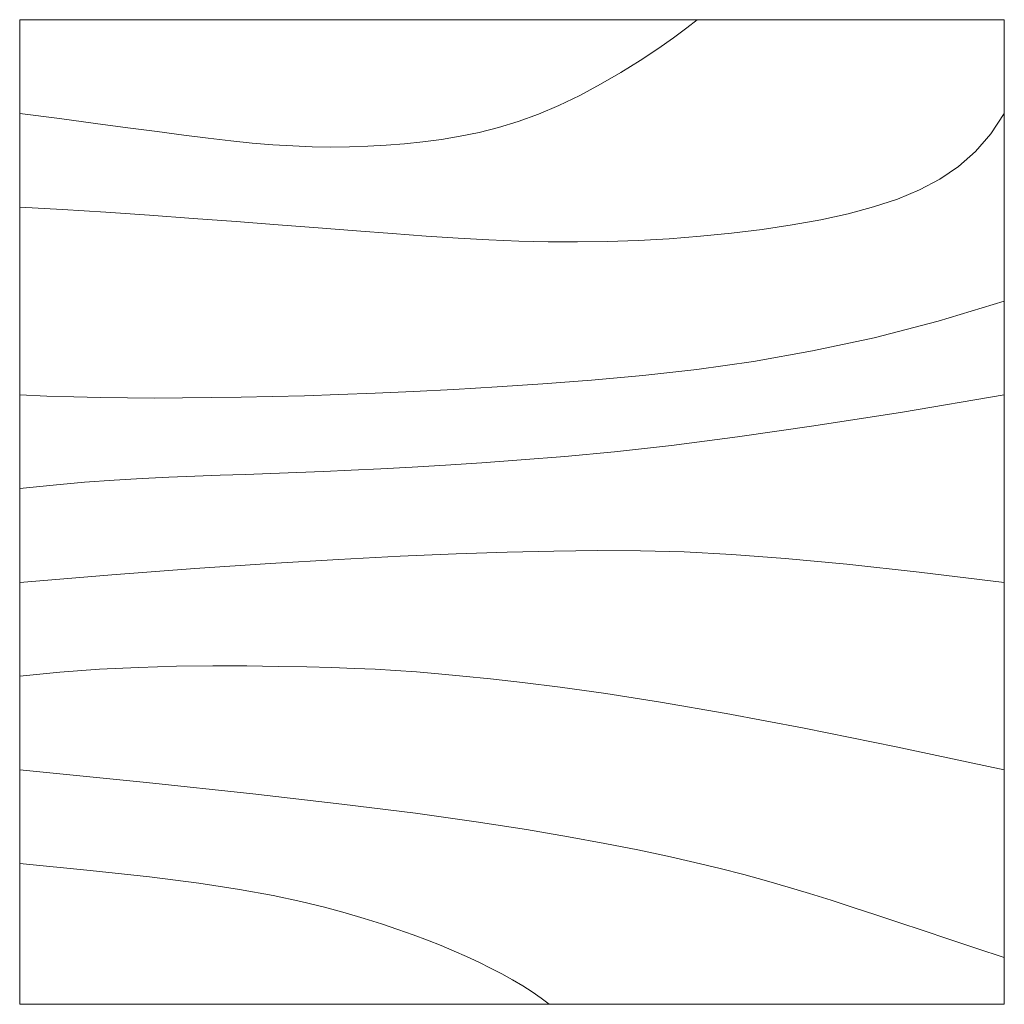
# Model space of a CAD drawing. Units: inches. Extents: x 19 to 15718, y 7 to 930.
# Tile 1 of 11: x 13723 to 13765, y 366 to 408. Entities that reach past the tile are written whole.
import ezdxf

# ---------------------------------------------------------------- set-up
doc = ezdxf.new("R2010")
doc.units = ezdxf.units.IN
doc.header["$MEASUREMENT"] = 0
doc.layers.add('A-FURN', color=8, linetype='Continuous', lineweight=18)

# ---------------------------------------------------------------- blocks, each defined once
blk = doc.blocks.new('Table - Square Woodgrain 42 x 42 in.')
blk.add_line((0, -42), (42, -42))
for points in [[(0, -4), (1.704, -4.2172), (3.2358, -4.4188), (4.615, -4.604), (5.8615, -4.7721), (6.9951, -4.9224), (8.0357, -5.0541), (9.0031, -5.1667), (9.9171, -5.2594), (10.7951, -5.3316), (11.6445, -5.3836), (12.4702, -5.4157), (13.277, -5.4283), (14.0698, -5.4217), (14.8535, -5.3964), (15.6331, -5.3526), (16.4133, -5.2908), (17.1986, -5.2103), (17.9913, -5.1062), (18.793, -4.9727), (19.6056, -4.8038), (20.4307, -4.5937), (21.2701, -4.3365), (22.1256, -4.0262), (22.9989, -3.6571), (23.888, -3.2272), (24.7756, -2.7516), (25.6408, -2.2491), (26.4624, -1.7387), (27.2195, -1.2395), (27.891, -0.7703), (28.456, -0.3501), (28.8934, 0.002)], [(0, -42), (0, 0), (42, 0), (42, -42)], [(0, -8), (1.8203, -8.1001), (3.6741, -8.2149), (5.5411, -8.3408), (7.4011, -8.4741), (9.2339, -8.6112), (11.0193, -8.7484), (12.7371, -8.8821), (14.3671, -9.0086), (15.8954, -9.1246), (17.3337, -9.2278), (18.6997, -9.3159), (20.0116, -9.387), (21.2871, -9.4389), (22.5442, -9.4696), (23.8008, -9.477), (25.0749, -9.459), (26.3791, -9.4137), (27.7049, -9.3403), (29.0383, -9.2382), (30.3655, -9.1068), (31.6728, -8.9455), (32.9461, -8.7535), (34.1717, -8.5304), (35.3358, -8.2756), (36.4268, -7.9863), (37.443, -7.6521), (38.3849, -7.2603), (39.253, -6.7986), (40.048, -6.2542), (40.7705, -5.6147), (41.421, -4.8674), (42, -4)], [(42, -12), (39.1784, -12.8621), (36.4519, -13.5654), (33.8246, -14.1294), (31.3004, -14.5731), (28.8832, -14.9161), (26.577, -15.1775), (24.3858, -15.3768), (22.3136, -15.5332), (20.3622, -15.6632), (18.5254, -15.7718), (16.7947, -15.8612), (15.1618, -15.9338), (13.6183, -15.9916), (12.1558, -16.0369), (10.7659, -16.0718), (9.4403, -16.0987), (8.1703, -16.1191), (6.9461, -16.1325), (5.7577, -16.1377), (4.595, -16.1335), (3.4479, -16.1188), (2.3064, -16.0924), (1.1604, -16.0532), (0, -16)], [(42, -16), (37.6529, -16.7365), (33.8802, -17.329), (30.6179, -17.7961), (27.8015, -18.1561), (25.3668, -18.4275), (23.2497, -18.6288), (21.3859, -18.7785), (19.7111, -18.8949), (18.1693, -18.9939), (16.7375, -19.0795), (15.401, -19.1534), (14.1449, -19.217), (12.9544, -19.2717), (11.8148, -19.3191), (10.7113, -19.3606), (9.6291, -19.3976), (8.5534, -19.4323), (7.47, -19.4689), (6.3643, -19.5122), (5.222, -19.5672), (4.0288, -19.6386), (2.7703, -19.7313), (1.4321, -19.8501), (0, -20)], [(0, -24), (3.9243, -23.6805), (7.4766, -23.4138), (10.6891, -23.1954), (13.5943, -23.0205), (16.2247, -22.8847), (18.6125, -22.7832), (20.7903, -22.7116), (22.7903, -22.6651), (24.6563, -22.642), (26.4764, -22.6507), (28.35, -22.7024), (30.3766, -22.8084), (32.6555, -22.98), (35.2861, -23.2283), (38.3678, -23.5645), (42, -24)], [(42, -32), (37.392, -31.017), (33.4585, -30.2231), (30.1291, -29.5949), (27.3334, -29.109), (25.0009, -28.742), (23.0612, -28.4707), (21.4439, -28.2716), (20.0786, -28.1215), (18.8998, -28.0002), (17.8609, -27.9014), (16.9206, -27.8219), (16.0371, -27.7588), (15.1691, -27.709), (14.2748, -27.6693), (13.3128, -27.6368), (12.2415, -27.6083), (11.0295, -27.5824), (9.6867, -27.5643), (8.233, -27.5608), (6.6884, -27.5787), (5.0728, -27.6248), (3.4062, -27.7058), (1.7086, -27.8286), (0, -28)], [(0, -32), (5.4026, -32.5358), (9.9494, -33.019), (13.7424, -33.4553), (16.8834, -33.8505), (19.4743, -34.2106), (21.6171, -34.5413), (23.4136, -34.8486), (24.9657, -35.1382), (26.3614, -35.4156), (27.6332, -35.6841), (28.7995, -35.9467), (29.8788, -36.2064), (30.8897, -36.4661), (31.8507, -36.7288), (32.7802, -36.9973), (33.6968, -37.2747), (34.6175, -37.5635), (35.5531, -37.8651), (36.5128, -38.1805), (37.506, -38.5108), (38.5421, -38.8568), (39.6302, -39.2197), (40.7797, -39.6004), (42, -40)], [(0, -36), (3.0098, -36.2857), (5.5354, -36.5643), (7.6368, -36.8359), (9.374, -37.1009), (10.807, -37.3597), (11.9957, -37.6126), (13.0002, -37.8599), (13.8804, -38.102), (14.6874, -38.3393), (15.4365, -38.5729), (16.1338, -38.8041), (16.7858, -39.0341), (17.3987, -39.264), (17.9787, -39.4952), (18.5322, -39.7288), (19.0655, -39.9662), (19.5832, -40.2081), (20.0842, -40.4544), (20.5657, -40.7046), (21.0249, -40.9581), (21.459, -41.2144), (21.8653, -41.4731), (22.2409, -41.7335), (22.5831, -41.9951)]]:
    blk.add_lwpolyline(points)

msp = doc.modelspace()

# ---------------------------------------------------------------- block references
at = {"layer": 'A-FURN'}
msp.add_blockref('Table - Square Woodgrain 42 x 42 in.', (13722.929, 408.407), dxfattribs=at)

doc.saveas('drawing.dxf')
